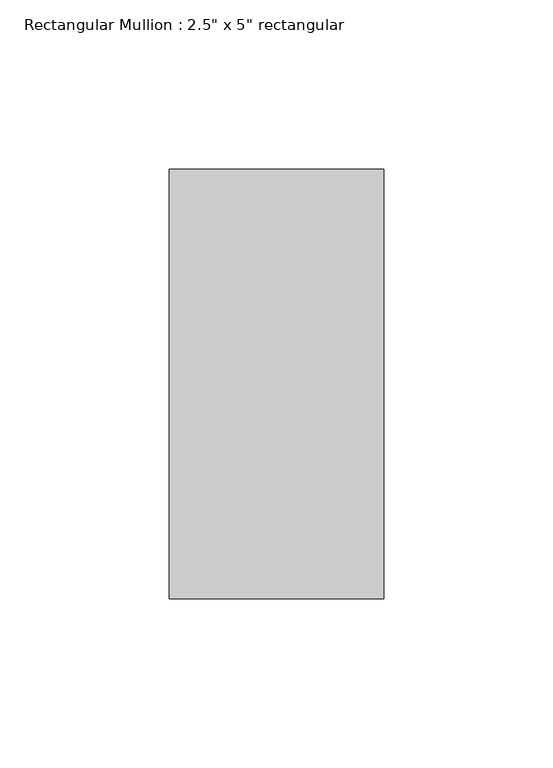
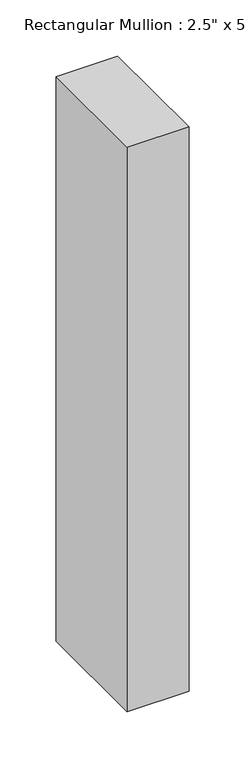
"""IFC4 building model written with IfcOpenShell, lengths in millimetres: member geometry."""

from ifc_helpers import new_model, si_unit, frame, origin, place, context, project, spatial, polyline, outline, extrude, source, transform, mapped, element, save


def member_94110371(model_context):
    return source(origin(), model_context, "Body", "SweptSolid", [
        extrude(outline(polyline([(0.0, 63.5), (0.0, -63.5), (-63.5, -63.5), (-63.5, 63.5), (0.0, 63.5)])), frame((0.0, 0.0, -613.8333333), z_axis=(0.0, 0.0, 1.0), x_axis=(1.0, 0.0, 0.0)), (0.0, 0.0, 1.0), 613.8333333),
    ])


if __name__ == "__main__":
    model = new_model("IFC4")
    model_context = context("Model", 3, world=origin())
    ifc_project = project(units=[si_unit("LENGTHUNIT", "METRE", prefix="MILLI")], contexts=[model_context])
    site = spatial("IfcSite", under=ifc_project)
    building = spatial("IfcBuilding", under=site)
    placement = place(None, origin())
    member_shape = member_94110371(model_context)
    element("IfcMember", 1, ObjectType="Rectangular Mullion : 2.5\" x 5\" rectangular", at=placement, inside=building, context=model_context, shape_type="MappedRepresentation", body=[
        mapped(member_shape, transform((0.0, 0.0, 0.0), x_axis=(1.0, 0.0, 0.0), y_axis=(0.0, 1.0, 0.0), z_axis=(0.0, 0.0, 1.0))),
    ])
    save(model, "model.ifc")

# Revit data of these elements
# Type "Rectangular Mullion : 2.5\" x 5\" rectangular"
#   built-in parameter 1007304 = 0.416667 (stored number, unit not read)
#   built-in parameter 1007301 = 0.104167 (stored number, unit not read)
#   built-in parameter 1007300 = 0.104167 (stored number, unit not read)
# Element 1 (IfcMember, "Rectangular Mullion : 2.5\" x 5\" rectangular")
#   Materials on its faces: "Aluminum"
# Materials
#   "Aluminum": class "Metal", colour RGB 247 247 247, transparency 0, Description = "Aluminum 6061", Cost = 0
